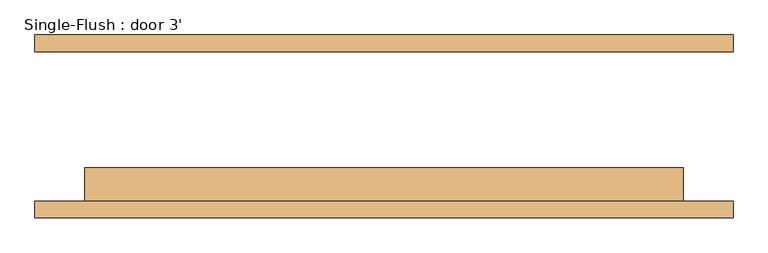
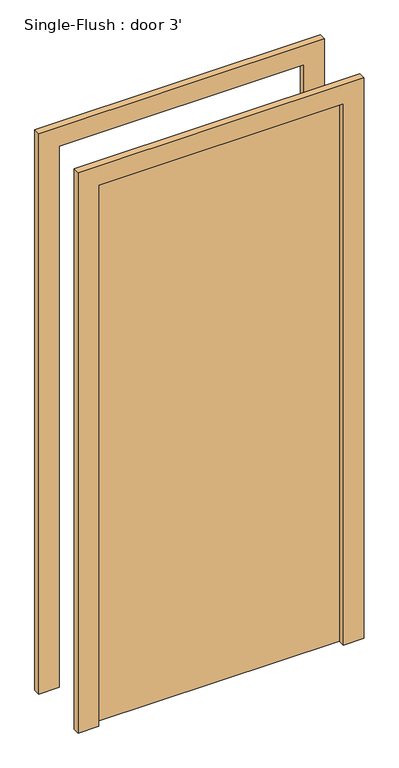
"""IFC4 building model written with IfcOpenShell, lengths in millimetres: door geometry, Single-Flush : door 3'."""

from ifc_helpers import new_model, si_unit, frame, origin, origin_with_axes, place, context, project, spatial, polyline, outline, extrude, source, transform, mapped, element, save


def single_flush_door_3_a90ba1ad(model_context):
    return source(origin(), model_context, "Body", "SweptSolid", [
        extrude(outline(polyline([(2209.8, -533.4), (0.0, -533.4), (0.0, -457.2), (2133.6, -457.2), (2133.6, 457.2), (0.0, 457.2), (0.0, 533.4), (2209.8, 533.4), (2209.8, -533.4)])), frame((0.0, -139.7, 0.0), z_axis=(0.0, 1.0, 0.0), x_axis=(0.0, 0.0, 1.0)), (0.0, 0.0, 1.0), 25.4),
        extrude(outline(polyline([(2209.8, 533.4), (2209.8, -533.4), (0.0, -533.4), (0.0, -457.2), (2133.6, -457.2), (2133.6, 457.2), (0.0, 457.2), (0.0, 533.4), (2209.8, 533.4)])), frame((0.0, 114.3, 0.0), z_axis=(0.0, 1.0, 0.0), x_axis=(0.0, 0.0, 1.0)), (0.0, 0.0, 1.0), 25.4),
        extrude(outline(polyline([(457.2, -63.5), (457.2, -114.3), (-457.2, -114.3), (-457.2, -63.5), (457.2, -63.5)])), origin_with_axes(), (0.0, 0.0, 1.0), 2133.6),
    ])


if __name__ == "__main__":
    model = new_model("IFC4")
    model_context = context("Model", 3, world=origin())
    ifc_project = project(units=[si_unit("LENGTHUNIT", "METRE", prefix="MILLI")], contexts=[model_context])
    site = spatial("IfcSite", under=ifc_project)
    building = spatial("IfcBuilding", under=site)
    placement = place(None, origin())
    single_flush_door_3_shape = single_flush_door_3_a90ba1ad(model_context)
    element("IfcDoor", 1, ObjectType="Single-Flush : door 3'", at=placement, inside=building, context=model_context, shape_type="MappedRepresentation", body=[
        mapped(single_flush_door_3_shape, transform((0.0, 0.0, 0.0), x_axis=(1.0, 0.0, 0.0), y_axis=(0.0, 1.0, 0.0), z_axis=(0.0, 0.0, 1.0))),
    ])
    save(model, "model.ifc")

# Revit data of these elements
# Type "Single-Flush : door 3'"
#   Type Mark = "8"
#   Construction Type Id = "MDOOR"
#   Assembly Code = "C1020"
#   Analytic Construction = "Metal"
#   Thickness = 0' - 2"
#   Heat Transfer Coefficient (U) = 0.651978 BTU/(h·ft²·°F)
#   Height = 7' - 0"
#   Trim Projection Ext = 0' - 1"
#   Trim Projection Int = 0' - 1"
#   Trim Width = 0' - 3"
#   Width = 3' - 0"
#   Define Thermal Properties by = 1
#   Door Material = Door - Panel
#   Frame Material = Door - Frame
#   Visual Light Transmittance = 0
#   Solar Heat Gain Coefficient = 0
#   Function = (empty or 0)
#   Wall Closure = (empty or 0)
# Element 1 (IfcDoor, "Single-Flush : door 3'")
#   Materials on its faces: "Door - Frame", "Door - Panel"
# Materials
#   "Door - Panel": class "Wood", colour RGB 210 159 95, transparency 0, Cost = 0
#   "Door - Frame": colour RGB 118 70 51, transparency 0, Cost = 0
